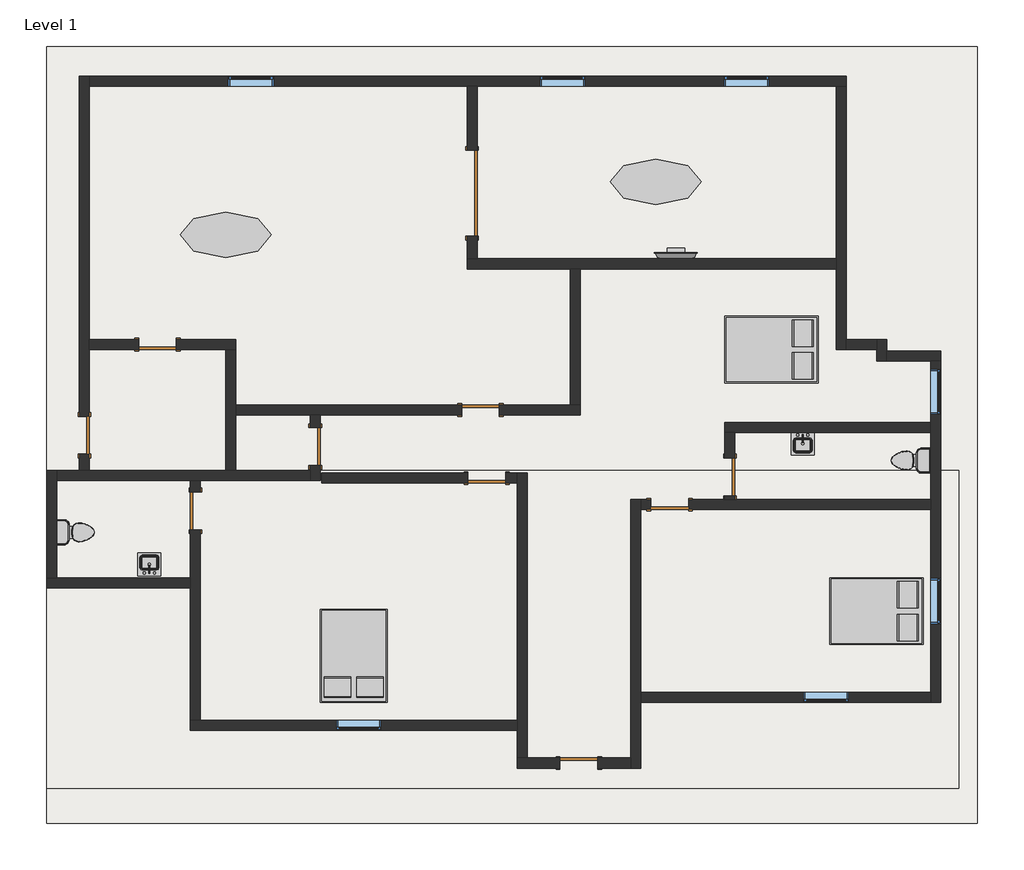
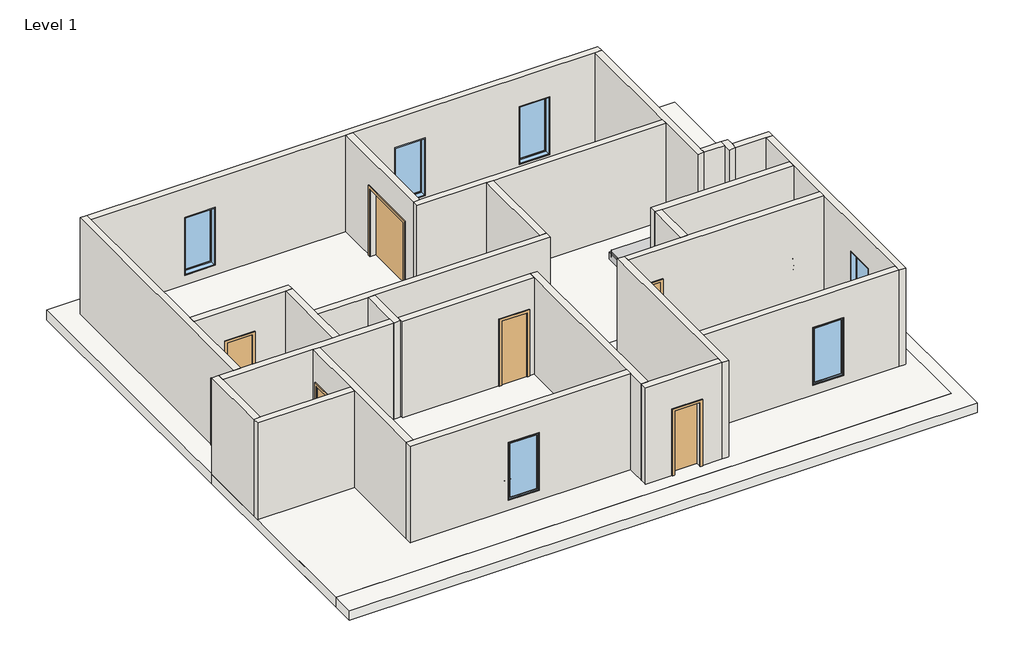
# One storey, incomplete: 27 walls, 10 doors, 7 windows, 6 furniture elements, 4 flow terminals, 3 slabs.
"""IFC4 building model written with IfcOpenShell, lengths in millimetres."""

from ifc_helpers import new_model, si_unit, frame, origin, origin_with_axes, place, context, project, spatial, polyline, outline, extrude, faceted_brep, transform, mapped, element, save
from components import door_f3de6620, door_53b1b562, door_fadea3f2, flow_terminal_871c2e40, toilet_domestic_3d_toilet_domestic_3d_f7549cf7, toilet_domestic_3d_toilet_domestic_3d_183bbd19, furniture_c8abb964, furniture_56245f3a, furniture_027a2ad9, window_9a779fa2, window_750da936

model = new_model("IFC4")

# Units and contexts
model_context = context("Model", 3, world=origin())
ifc_project = project(units=[si_unit("LENGTHUNIT", "METRE", prefix="MILLI")], contexts=[model_context])

# Site, building, storey
site = spatial("IfcSite", under=ifc_project)
building = spatial("IfcBuilding", under=site)
storey = spatial("IfcBuildingStorey", under=building, Name="Level 1", Elevation=0.0)

# Doors
placement = place(None, origin())
door_shape = door_f3de6620(model_context)
element("IfcDoor", 1, ObjectType="Door-Double-Flush_Panel-Double-Acting : 68\" x 84\"", at=placement, inside=storey, context=model_context, shape_type="MappedRepresentation", body=[
    mapped(door_shape, transform((-10205.5126434, 12193.5007235, 0.0), x_axis=(0.0, -1.0, 0.0), y_axis=(1.0, 0.0, 0.0), z_axis=(0.0, 0.0, 1.0))),
])
door_2_shape = door_53b1b562(model_context)
element("IfcDoor", 2, ObjectType="Single-Flush : 30\" x 80\"", at=placement, inside=storey, context=model_context, shape_type="MappedRepresentation", body=[
    mapped(door_2_shape, transform((-16538.7421908, 9145.5007235, 0.0), x_axis=(1.0, 0.0, 0.0), y_axis=(0.0, 1.0, 0.0), z_axis=(0.0, 0.0, 1.0))),
])
element("IfcDoor", 3, ObjectType="Single-Flush : 30\" x 80\"", at=placement, inside=storey, context=model_context, shape_type="MappedRepresentation", body=[
    mapped(door_2_shape, transform((-18011.9421908, 7316.7007235, 0.0), x_axis=(0.0, 1.0, 0.0), y_axis=(-1.0, 0.0, 0.0), z_axis=(0.0, 0.0, 1.0))),
])
element("IfcDoor", 4, ObjectType="Single-Flush : 30\" x 80\"", at=placement, inside=storey, context=model_context, shape_type="MappedRepresentation", body=[
    mapped(door_2_shape, transform((-9909.3421908, 6453.1007235, 0.0), x_axis=(1.0, 0.0, 0.0), y_axis=(0.0, 1.0, 0.0), z_axis=(0.0, 0.0, 1.0))),
])
element("IfcDoor", 5, ObjectType="Single-Flush : 30\" x 80\"", at=placement, inside=storey, context=model_context, shape_type="MappedRepresentation", body=[
    mapped(door_2_shape, transform((-8055.1421908, 712.7007235, 0.0), x_axis=(-1.0, 0.0, 0.0), y_axis=(0.0, -1.0, 0.0), z_axis=(0.0, 0.0, 1.0))),
])
door_3_shape = door_fadea3f2(model_context)
element("IfcDoor", 6, ObjectType="Single-Flush : 30\" x 80\"", at=placement, inside=storey, context=model_context, shape_type="MappedRepresentation", body=[
    mapped(door_3_shape, transform((-15776.7421908, 5792.7007235, 0.0), x_axis=(0.0, 1.0, 0.0), y_axis=(-1.0, 0.0, 0.0), z_axis=(0.0, 0.0, 1.0))),
])
element("IfcDoor", 7, ObjectType="Single-Flush : 30\" x 80\"", at=placement, inside=storey, context=model_context, shape_type="MappedRepresentation", body=[
    mapped(door_3_shape, transform((-13363.7421908, 7088.1007235, 0.0), x_axis=(0.0, -1.0, 0.0), y_axis=(1.0, 0.0, 0.0), z_axis=(0.0, 0.0, 1.0))),
])
element("IfcDoor", 8, ObjectType="Single-Flush : 30\" x 80\"", at=placement, inside=storey, context=model_context, shape_type="MappedRepresentation", body=[
    mapped(door_3_shape, transform((-10036.3421908, 7824.7007235, 0.0), x_axis=(1.0, 0.0, 0.0), y_axis=(0.0, 1.0, 0.0), z_axis=(0.0, 0.0, 1.0))),
])
element("IfcDoor", 9, ObjectType="Single-Flush : 30\" x 80\"", at=placement, inside=storey, context=model_context, shape_type="MappedRepresentation", body=[
    mapped(door_3_shape, transform((-6226.3421908, 5919.7007235, 0.0), x_axis=(-1.0, 0.0, 0.0), y_axis=(0.0, -1.0, 0.0), z_axis=(0.0, 0.0, 1.0))),
])
element("IfcDoor", 10, ObjectType="Single-Flush : 30\" x 80\"", at=placement, inside=storey, context=model_context, shape_type="MappedRepresentation", body=[
    mapped(door_3_shape, transform((-5014.2099629, 6478.5007235, 0.0), x_axis=(0.0, -1.0, 0.0), y_axis=(1.0, 0.0, 0.0), z_axis=(0.0, 0.0, 1.0))),
])

# Flow terminals
flow_terminal_shape = flow_terminal_871c2e40(model_context)
element("IfcFlowTerminal", 11, ObjectType="Sink Kitchen-Island : 18\" x 18\"", at=placement, inside=storey, context=model_context, shape_type="MappedRepresentation", body=[
    mapped(flow_terminal_shape, transform((-16688.1529503, 4715.5461246, 0.0), x_axis=(-1.0000000000000004, 0.0, 0.0), y_axis=(0.0, -1.0000000000000004, 0.0), z_axis=(0.0, 0.0, 1.0))),
])
element("IfcFlowTerminal", 12, ObjectType="Sink Kitchen-Island : 18\" x 18\"", at=placement, inside=storey, context=model_context, shape_type="MappedRepresentation", body=[
    mapped(flow_terminal_shape, transform((-3562.3314314, 7149.2553224, 0.0), x_axis=(1.0, 0.0, 0.0), y_axis=(0.0, 1.0, 0.0), z_axis=(0.0, 0.0, 1.0))),
])
toilet_domestic_3d_toilet_domestic_3d_shape = toilet_domestic_3d_toilet_domestic_3d_f7549cf7(model_context)
toilet_domestic_3d_toilet_domestic_3d_2_shape = toilet_domestic_3d_toilet_domestic_3d_183bbd19(model_context)
element("IfcFlowTerminal", 13, ObjectType="Toilet-Domestic-3D : Toilet-Domestic-3D", at=placement, inside=storey, context=model_context, shape_type="MappedRepresentation", body=[
    mapped(toilet_domestic_3d_toilet_domestic_3d_shape, transform((-18113.5421908, 5360.9007235, 0.0), x_axis=(0.0, 1.0000000000000002, 0.0), y_axis=(-1.0000000000000002, 0.0, 0.0), z_axis=(0.0, 0.0, 1.0))),
    mapped(toilet_domestic_3d_toilet_domestic_3d_2_shape, transform((-18113.5421908, 5360.9007235, 0.0), x_axis=(0.0, 1.0000000000000002, 0.0), y_axis=(-1.0000000000000002, 0.0, 0.0), z_axis=(0.0, 0.0, 1.0))),
])
element("IfcFlowTerminal", 14, ObjectType="Toilet-Domestic-3D : Toilet-Domestic-3D", at=placement, inside=storey, context=model_context, shape_type="MappedRepresentation", body=[
    mapped(toilet_domestic_3d_toilet_domestic_3d_shape, transform((-1463.2382182, 6808.7007235, 0.0), x_axis=(0.0, -1.0000000000000004, 0.0), y_axis=(1.0000000000000004, 0.0, 0.0), z_axis=(0.0, 0.0, 1.0))),
    mapped(toilet_domestic_3d_toilet_domestic_3d_2_shape, transform((-1463.2382182, 6808.7007235, 0.0), x_axis=(0.0, -1.0000000000000004, 0.0), y_axis=(1.0000000000000004, 0.0, 0.0), z_axis=(0.0, 0.0, 1.0))),
])

# Furniture
furniture_shape = furniture_c8abb964(model_context)
element("IfcFurniture", 15, ObjectType="Bed-Box : Double 53\" x 74\"", at=placement, inside=storey, context=model_context, shape_type="MappedRepresentation", body=[
    mapped(furniture_shape, transform((-12249.8897318, 2637.2712153, 0.0), x_axis=(-0.9999999999999999, 0.0, 0.0), y_axis=(0.0, -0.9999999999999999, 0.0), z_axis=(0.0, 0.0, 1.0))),
])
element("IfcFurniture", 16, ObjectType="Bed-Box : Double 53\" x 74\"", at=placement, inside=storey, context=model_context, shape_type="MappedRepresentation", body=[
    mapped(furniture_shape, transform((-1826.3126826, 4112.5531825, 0.0), x_axis=(0.0, -1.0000000000000002, 0.0), y_axis=(1.0000000000000002, 0.0, 0.0), z_axis=(0.0, 0.0, 1.0))),
])
element("IfcFurniture", 17, ObjectType="Bed-Box : Double 53\" x 74\"", at=placement, inside=storey, context=model_context, shape_type="MappedRepresentation", body=[
    mapped(furniture_shape, transform((-3941.5804547, 9383.0531825, 0.0), x_axis=(0.0, -0.9999999999999998, 0.0), y_axis=(0.9999999999999998, 0.0, 0.0), z_axis=(0.0, 0.0, 1.0))),
])
furniture_2_shape = furniture_56245f3a(model_context)
element("IfcFurniture", 18, ObjectType="TV - Flat Screen : 32\"", at=placement, inside=storey, context=model_context, shape_type="MappedRepresentation", body=[
    mapped(furniture_2_shape, transform((-6103.286705, 10931.2393472, 914.4), x_axis=(-0.9999999999999998, 0.0, 0.0), y_axis=(0.0, -0.9999999999999998, 0.0), z_axis=(0.0, 0.0, 1.0))),
])
furniture_3_shape = furniture_027a2ad9(model_context)
element("IfcFurniture", 19, ObjectType="Table-Ellipse : 72\" x 36\"", at=placement, inside=storey, context=model_context, shape_type="MappedRepresentation", body=[
    mapped(furniture_3_shape, transform((-15167.1421908, 11355.3007235, 0.0), x_axis=(1.0, 0.0, 0.0), y_axis=(0.0, 1.0, 0.0), z_axis=(0.0, 0.0, 1.0))),
])
element("IfcFurniture", 20, ObjectType="Table-Ellipse : 72\" x 36\"", at=placement, inside=storey, context=model_context, shape_type="MappedRepresentation", body=[
    mapped(furniture_3_shape, transform((-6505.7421908, 12422.1007235, 0.0), x_axis=(1.0, 0.0, 0.0), y_axis=(0.0, 1.0, 0.0), z_axis=(0.0, 0.0, 1.0))),
])

# Slabs
element("IfcSlab", 21, ObjectType="Generic - 12\"", at=placement, inside=storey, context=model_context, shape_type="SweptSolid", body=[
    extrude(outline(polyline([(-765.3421908, 14555.7007235), (-765.3421908, 6021.3007235), (-18113.5421908, 6021.3007235), (-18113.5421908, 14555.7007235), (-765.3421908, 14555.7007235)])), frame((0.0, 0.0, -304.8), z_axis=(0.0, 0.0, 1.0), x_axis=(1.0, 0.0, 0.0)), (0.0, 0.0, 1.0), 304.8),
])
element("IfcSlab", 22, ObjectType="Generic - 12\"", at=placement, inside=storey, context=model_context, shape_type="SweptSolid", body=[
    extrude(outline(polyline([(-409.7421908, 6605.5007235), (-409.7421908, 204.7007235), (-18773.9421908, 204.7007235), (-18773.9421908, 6605.5007235), (-409.7421908, 6605.5007235)])), frame((0.0, 0.0, -304.8), z_axis=(0.0, 0.0, 1.0), x_axis=(1.0, 0.0, 0.0)), (0.0, 0.0, 1.0), 304.8),
])
element("IfcSlab", 23, ObjectType="Generic - 12\"", at=placement, inside=storey, context=model_context, shape_type="SweptSolid", body=[
    extrude(outline(polyline([(-28.7421908, 15149.4135016), (-28.7421908, -496.9864984), (-18773.9421908, -496.9864984), (-18773.9421908, 15149.4135016), (-28.7421908, 15149.4135016)])), frame((0.0, 0.0, -304.8), z_axis=(0.0, 0.0, 1.0), x_axis=(1.0, 0.0, 0.0)), (0.0, 0.0, 1.0), 304.8),
])

# Walls
element("IfcWall", 24, ObjectType="Generic - 8\"", at=placement, inside=storey, context=model_context, shape_type="Brep", body=[
    faceted_brep([(-17910.3421908, 7697.7007235, 2032.0), (-17910.3421908, 7697.7007235, 0.0), (-17910.3421908, 9043.9007235, 0.0), (-17910.3421908, 9247.1007235, 0.0), (-17910.3421908, 14352.5007235, 0.0), (-17910.3421908, 14555.7007235, 0.0), (-17910.3421908, 14555.7007235, 3048.0), (-17910.3421908, 14352.5007235, 3048.0), (-17910.3421908, 9247.1007235, 3048.0), (-17910.3421908, 9043.9007235, 3048.0), (-17910.3421908, 6605.5007235, 3048.0), (-17910.3421908, 6605.5007235, 0.0), (-17910.3421908, 6935.7007235, 0.0), (-17910.3421908, 6935.7007235, 2032.0), (-18113.5421908, 14555.7007235, 0.0), (-18113.5421908, 7697.7007235, 0.0), (-18113.5421908, 7697.7007235, 2032.0), (-18113.5421908, 6935.7007235, 2032.0), (-18113.5421908, 6935.7007235, 0.0), (-18113.5421908, 6605.5007235, 0.0), (-18113.5421908, 6605.5007235, 3048.0), (-18113.5421908, 14555.7007235, 3048.0)], [[[0, 1, 2, 3, 4, 5, 6, 7, 8, 9, 10, 11, 12, 13]], [[14, 15, 16, 17, 18, 19, 20, 21]], [[12, 11, 19, 18]], [[5, 4, 3, 2, 1, 15, 14]], [[6, 5, 14, 21]], [[11, 10, 20, 19]], [[16, 15, 1, 0]], [[17, 16, 0, 13]], [[18, 17, 13, 12]], [[10, 9, 8, 7, 6, 21, 20]]]),
])
element("IfcWall", 25, ObjectType="Generic - 8\"", at=placement, inside=storey, context=model_context, shape_type="Brep", body=[
    faceted_brep([(-17910.3421908, 14352.5007235, 0.0), (-10307.1126434, 14352.5007235, 0.0), (-10103.9126434, 14352.5007235, 0.0), (-2873.5421908, 14352.5007235, 0.0), (-2670.3421908, 14352.5007235, 0.0), (-2670.3421908, 14352.5007235, 3048.0), (-2873.5421908, 14352.5007235, 3048.0), (-10103.9126434, 14352.5007235, 3048.0), (-10307.1126434, 14352.5007235, 3048.0), (-17910.3421908, 14352.5007235, 3048.0), (-14201.9421908, 14352.5007235, 2133.6), (-14201.9421908, 14352.5007235, 304.8), (-15116.3421908, 14352.5007235, 304.8), (-15116.3421908, 14352.5007235, 2133.6), (-8842.5421908, 14352.5007235, 2133.6), (-7928.1421908, 14352.5007235, 2133.6), (-7928.1421908, 14352.5007235, 304.8), (-8842.5421908, 14352.5007235, 304.8), (-4219.7421908, 14352.5007235, 2133.6), (-4219.7421908, 14352.5007235, 304.8), (-5134.1421908, 14352.5007235, 304.8), (-5134.1421908, 14352.5007235, 2133.6), (-17910.3421908, 14555.7007235, 0.0), (-17910.3421908, 14555.7007235, 3048.0), (-2670.3421908, 14555.7007235, 3048.0), (-2670.3421908, 14555.7007235, 0.0), (-14201.9421908, 14555.7007235, 2133.6), (-15116.3421908, 14555.7007235, 2133.6), (-15116.3421908, 14555.7007235, 304.8), (-14201.9421908, 14555.7007235, 304.8), (-8842.5421908, 14555.7007235, 2133.6), (-8842.5421908, 14555.7007235, 304.8), (-7928.1421908, 14555.7007235, 304.8), (-7928.1421908, 14555.7007235, 2133.6), (-4219.7421908, 14555.7007235, 2133.6), (-5134.1421908, 14555.7007235, 2133.6), (-5134.1421908, 14555.7007235, 304.8), (-4219.7421908, 14555.7007235, 304.8)], [[[0, 1, 2, 3, 4, 5, 6, 7, 8, 9], [10, 11, 12, 13], [14, 15, 16, 17], [18, 19, 20, 21]], [[22, 23, 24, 25], [26, 27, 28, 29], [30, 31, 32, 33], [34, 35, 36, 37]], [[4, 3, 2, 1, 0, 22, 25]], [[0, 9, 23, 22]], [[5, 4, 25, 24]], [[11, 10, 26, 29]], [[12, 11, 29, 28]], [[13, 12, 28, 27]], [[10, 13, 27, 26]], [[31, 30, 14, 17]], [[32, 31, 17, 16]], [[33, 32, 16, 15]], [[30, 33, 15, 14]], [[19, 18, 34, 37]], [[20, 19, 37, 36]], [[21, 20, 36, 35]], [[18, 21, 35, 34]], [[9, 8, 7, 6, 5, 24, 23]]]),
])
element("IfcWall", 26, ObjectType="Generic - 8\"", at=placement, inside=storey, context=model_context, shape_type="Brep", body=[
    faceted_brep([(-2873.5421908, 14352.5007235, 0.0), (-2873.5421908, 10872.7007235, 0.0), (-2873.5421908, 10669.5007235, 0.0), (-2873.5421908, 9043.9007235, 0.0), (-2873.5421908, 9043.9007235, 3048.0), (-2873.5421908, 10669.5007235, 3048.0), (-2873.5421908, 10872.7007235, 3048.0), (-2873.5421908, 14352.5007235, 3048.0), (-2670.3421908, 14352.5007235, 0.0), (-2670.3421908, 14352.5007235, 3048.0), (-2670.3421908, 9247.1007235, 3048.0), (-2670.3421908, 9043.9007235, 3048.0), (-2670.3421908, 9043.9007235, 0.0), (-2670.3421908, 9247.1007235, 0.0)], [[[0, 1, 2, 3, 4, 5, 6, 7]], [[8, 9, 10, 11, 12, 13]], [[3, 2, 1, 0, 8, 13, 12]], [[0, 7, 9, 8]], [[4, 3, 12, 11]], [[7, 6, 5, 4, 11, 10, 9]]]),
])
element("IfcWall", 27, ObjectType="Generic - 8\"", at=placement, inside=storey, context=model_context, shape_type="SweptSolid", body=[
    extrude(outline(polyline([(-2060.7421908, 9043.9007235), (-2670.3421908, 9043.9007235), (-2670.3421908, 9247.1007235), (-2060.7421908, 9247.1007235), (-2060.7421908, 9043.9007235)])), origin_with_axes(), (0.0, 0.0, 1.0), 3048.0),
])
element("IfcWall", 28, ObjectType="Generic - 8\"", at=placement, inside=storey, context=model_context, shape_type="Brep", body=[
    faceted_brep([(-2060.7421908, 9247.1007235, 0.0), (-2060.7421908, 9043.9007235, 0.0), (-2060.7421908, 8815.3007235, 0.0), (-2060.7421908, 8815.3007235, 3048.0), (-2060.7421908, 9043.9007235, 3048.0), (-2060.7421908, 9247.1007235, 3048.0), (-1857.5421908, 9247.1007235, 0.0), (-1857.5421908, 9247.1007235, 3048.0), (-1857.5421908, 9018.5007235, 3048.0), (-1857.5421908, 8815.3007235, 3048.0), (-1857.5421908, 8815.3007235, 0.0), (-1857.5421908, 9018.5007235, 0.0)], [[[0, 1, 2, 3, 4, 5]], [[6, 7, 8, 9, 10, 11]], [[2, 1, 0, 6, 11, 10]], [[0, 5, 7, 6]], [[3, 2, 10, 9]], [[5, 4, 3, 9, 8, 7]]]),
])
element("IfcWall", 29, ObjectType="Generic - 8\"", at=placement, inside=storey, context=model_context, shape_type="Brep", body=[
    faceted_brep([(-1857.5421908, 8815.3007235, 0.0), (-968.5421908, 8815.3007235, 0.0), (-765.3421908, 8815.3007235, 0.0), (-765.3421908, 8815.3007235, 3048.0), (-968.5421908, 8815.3007235, 3048.0), (-1857.5421908, 8815.3007235, 3048.0), (-1857.5421908, 9018.5007235, 0.0), (-1857.5421908, 9018.5007235, 3048.0), (-765.3421908, 9018.5007235, 3048.0), (-765.3421908, 9018.5007235, 0.0)], [[[0, 1, 2, 3, 4, 5]], [[6, 7, 8, 9]], [[2, 1, 0, 6, 9]], [[0, 5, 7, 6]], [[3, 2, 9, 8]], [[5, 4, 3, 8, 7]]]),
])
element("IfcWall", 30, ObjectType="Generic - 8\"", at=placement, inside=storey, context=model_context, shape_type="Brep", body=[
    faceted_brep([(-968.5421908, 8815.3007235, 0.0), (-968.5421908, 7570.7007235, 0.0), (-968.5421908, 7367.5007235, 0.0), (-968.5421908, 6021.3007235, 0.0), (-968.5421908, 5818.1007235, 0.0), (-968.5421908, 2135.1007235, 0.0), (-968.5421908, 1931.9007235, 0.0), (-968.5421908, 1931.9007235, 3048.0), (-968.5421908, 2135.1007235, 3048.0), (-968.5421908, 5818.1007235, 3048.0), (-968.5421908, 6021.3007235, 3048.0), (-968.5421908, 7367.5007235, 3048.0), (-968.5421908, 7570.7007235, 3048.0), (-968.5421908, 8815.3007235, 3048.0), (-968.5421908, 7735.8007235, 2133.6), (-968.5421908, 7735.8007235, 304.8), (-968.5421908, 8650.2007235, 304.8), (-968.5421908, 8650.2007235, 2133.6), (-968.5421908, 3519.4007235, 2133.6), (-968.5421908, 3519.4007235, 304.8), (-968.5421908, 4433.8007235, 304.8), (-968.5421908, 4433.8007235, 2133.6), (-765.3421908, 8815.3007235, 0.0), (-765.3421908, 8815.3007235, 3048.0), (-765.3421908, 1931.9007235, 3048.0), (-765.3421908, 1931.9007235, 0.0), (-765.3421908, 7735.8007235, 2133.6), (-765.3421908, 8650.2007235, 2133.6), (-765.3421908, 8650.2007235, 304.8), (-765.3421908, 7735.8007235, 304.8), (-765.3421908, 3519.4007235, 2133.6), (-765.3421908, 4433.8007235, 2133.6), (-765.3421908, 4433.8007235, 304.8), (-765.3421908, 3519.4007235, 304.8)], [[[0, 1, 2, 3, 4, 5, 6, 7, 8, 9, 10, 11, 12, 13], [14, 15, 16, 17], [18, 19, 20, 21]], [[22, 23, 24, 25], [26, 27, 28, 29], [30, 31, 32, 33]], [[6, 5, 4, 3, 2, 1, 0, 22, 25]], [[0, 13, 23, 22]], [[7, 6, 25, 24]], [[15, 14, 26, 29]], [[16, 15, 29, 28]], [[17, 16, 28, 27]], [[14, 17, 27, 26]], [[19, 18, 30, 33]], [[20, 19, 33, 32]], [[21, 20, 32, 31]], [[18, 21, 31, 30]], [[13, 12, 11, 10, 9, 8, 7, 24, 23]]]),
])
element("IfcWall", 31, ObjectType="Generic - 8\"", at=placement, inside=storey, context=model_context, shape_type="SweptSolid", body=[
    extrude(outline(polyline([(0.0, -968.5421908), (3048.0, -968.5421908), (3048.0, -6810.5421908), (0.0, -6810.5421908), (0.0, -968.5421908)]), holes=[polyline([(2133.6, -3533.9421908), (2133.6, -2619.5421908), (304.8, -2619.5421908), (304.8, -3533.9421908), (2133.6, -3533.9421908)])]), frame((0.0, 1931.9007235, 0.0), z_axis=(0.0, 1.0, 0.0), x_axis=(0.0, 0.0, 1.0)), (0.0, 0.0, 1.0), 203.2),
])
element("IfcWall", 32, ObjectType="Generic - 8\"", at=placement, inside=storey, context=model_context, shape_type="Brep", body=[
    faceted_brep([(-7013.7421908, 6021.3007235, 0.0), (-7013.7421908, 814.3007235, 0.0), (-7013.7421908, 611.1007235, 0.0), (-7013.7421908, 611.1007235, 3048.0), (-7013.7421908, 814.3007235, 3048.0), (-7013.7421908, 6021.3007235, 3048.0), (-6810.5421908, 6021.3007235, 0.0), (-6810.5421908, 6021.3007235, 3048.0), (-6810.5421908, 5818.1007235, 3048.0), (-6810.5421908, 2135.1007235, 3048.0), (-6810.5421908, 1931.9007235, 3048.0), (-6810.5421908, 611.1007235, 3048.0), (-6810.5421908, 611.1007235, 0.0), (-6810.5421908, 1931.9007235, 0.0), (-6810.5421908, 2135.1007235, 0.0), (-6810.5421908, 5818.1007235, 0.0)], [[[0, 1, 2, 3, 4, 5]], [[6, 7, 8, 9, 10, 11, 12, 13, 14, 15]], [[2, 1, 0, 6, 15, 14, 13, 12]], [[3, 2, 12, 11]], [[0, 5, 7, 6]], [[5, 4, 3, 11, 10, 9, 8, 7]]]),
])
element("IfcWall", 33, ObjectType="Generic - 8\"", at=placement, inside=storey, context=model_context, shape_type="Brep", body=[
    faceted_brep([(-8436.1421908, 814.3007235, 2032.0), (-8436.1421908, 814.3007235, 0.0), (-9096.5421908, 814.3007235, 0.0), (-9299.7421908, 814.3007235, 0.0), (-9299.7421908, 814.3007235, 3048.0), (-9096.5421908, 814.3007235, 3048.0), (-7013.7421908, 814.3007235, 3048.0), (-7013.7421908, 814.3007235, 0.0), (-7674.1421908, 814.3007235, 0.0), (-7674.1421908, 814.3007235, 2032.0), (-9299.7421908, 611.1007235, 0.0), (-8436.1421908, 611.1007235, 0.0), (-8436.1421908, 611.1007235, 2032.0), (-7674.1421908, 611.1007235, 2032.0), (-7674.1421908, 611.1007235, 0.0), (-7013.7421908, 611.1007235, 0.0), (-7013.7421908, 611.1007235, 3048.0), (-9299.7421908, 611.1007235, 3048.0)], [[[0, 1, 2, 3, 4, 5, 6, 7, 8, 9]], [[10, 11, 12, 13, 14, 15, 16, 17]], [[8, 7, 15, 14]], [[3, 2, 1, 11, 10]], [[7, 6, 16, 15]], [[4, 3, 10, 17]], [[12, 11, 1, 0]], [[13, 12, 0, 9]], [[14, 13, 9, 8]], [[6, 5, 4, 17, 16]]]),
])
element("IfcWall", 34, ObjectType="Generic - 8\"", at=placement, inside=storey, context=model_context, shape_type="Brep", body=[
    faceted_brep([(-9096.5421908, 814.3007235, 0.0), (-9096.5421908, 6554.7007235, 0.0), (-9096.5421908, 6554.7007235, 3048.0), (-9096.5421908, 814.3007235, 3048.0), (-9299.7421908, 814.3007235, 0.0), (-9299.7421908, 814.3007235, 3048.0), (-9299.7421908, 1373.1007235, 3048.0), (-9299.7421908, 1576.3007235, 3048.0), (-9299.7421908, 6351.5007235, 3048.0), (-9299.7421908, 6554.7007235, 3048.0), (-9299.7421908, 6554.7007235, 0.0), (-9299.7421908, 6351.5007235, 0.0), (-9299.7421908, 1576.3007235, 0.0), (-9299.7421908, 1373.1007235, 0.0)], [[[0, 1, 2, 3]], [[4, 5, 6, 7, 8, 9, 10, 11, 12, 13]], [[1, 0, 4, 13, 12, 11, 10]], [[0, 3, 5, 4]], [[2, 1, 10, 9]], [[3, 2, 9, 8, 7, 6, 5]]]),
])
element("IfcWall", 35, ObjectType="Generic - 8\"", at=placement, inside=storey, context=model_context, shape_type="Brep", body=[
    faceted_brep([(-9299.7421908, 1576.3007235, 0.0), (-15675.1421908, 1576.3007235, 0.0), (-15878.3421908, 1576.3007235, 0.0), (-15878.3421908, 1576.3007235, 3048.0), (-15675.1421908, 1576.3007235, 3048.0), (-9299.7421908, 1576.3007235, 3048.0), (-12944.6421908, 1576.3007235, 2133.6), (-12944.6421908, 1576.3007235, 304.8), (-12030.2421908, 1576.3007235, 304.8), (-12030.2421908, 1576.3007235, 2133.6), (-9299.7421908, 1373.1007235, 0.0), (-9299.7421908, 1373.1007235, 3048.0), (-15878.3421908, 1373.1007235, 3048.0), (-15878.3421908, 1373.1007235, 0.0), (-12944.6421908, 1373.1007235, 2133.6), (-12030.2421908, 1373.1007235, 2133.6), (-12030.2421908, 1373.1007235, 304.8), (-12944.6421908, 1373.1007235, 304.8)], [[[0, 1, 2, 3, 4, 5], [6, 7, 8, 9]], [[10, 11, 12, 13], [14, 15, 16, 17]], [[2, 1, 0, 10, 13]], [[0, 5, 11, 10]], [[3, 2, 13, 12]], [[7, 6, 14, 17]], [[8, 7, 17, 16]], [[9, 8, 16, 15]], [[6, 9, 15, 14]], [[5, 4, 3, 12, 11]]]),
])
element("IfcWall", 36, ObjectType="Generic - 8\"", at=placement, inside=storey, context=model_context, shape_type="Brep", body=[
    faceted_brep([(-15675.1421908, 6173.7007235, 2032.0), (-15675.1421908, 6173.7007235, 0.0), (-15675.1421908, 6402.3007235, 0.0), (-15675.1421908, 6402.3007235, 3048.0), (-15675.1421908, 1576.3007235, 3048.0), (-15675.1421908, 1576.3007235, 0.0), (-15675.1421908, 5411.7007235, 0.0), (-15675.1421908, 5411.7007235, 2032.0), (-15878.3421908, 6402.3007235, 0.0), (-15878.3421908, 6173.7007235, 0.0), (-15878.3421908, 6173.7007235, 2032.0), (-15878.3421908, 5411.7007235, 2032.0), (-15878.3421908, 5411.7007235, 0.0), (-15878.3421908, 4446.5007235, 0.0), (-15878.3421908, 4243.3007235, 0.0), (-15878.3421908, 1576.3007235, 0.0), (-15878.3421908, 1576.3007235, 3048.0), (-15878.3421908, 4243.3007235, 3048.0), (-15878.3421908, 4446.5007235, 3048.0), (-15878.3421908, 6402.3007235, 3048.0)], [[[0, 1, 2, 3, 4, 5, 6, 7]], [[8, 9, 10, 11, 12, 13, 14, 15, 16, 17, 18, 19]], [[6, 5, 15, 14, 13, 12]], [[2, 1, 9, 8]], [[5, 4, 16, 15]], [[3, 2, 8, 19]], [[10, 9, 1, 0]], [[11, 10, 0, 7]], [[12, 11, 7, 6]], [[4, 3, 19, 18, 17, 16]]]),
])
element("IfcWall", 37, ObjectType="Generic - 8\"", at=placement, inside=storey, context=model_context, shape_type="Brep", body=[
    faceted_brep([(-15878.3421908, 4446.5007235, 0.0), (-18570.7421908, 4446.5007235, 0.0), (-18773.9421908, 4446.5007235, 0.0), (-18773.9421908, 4446.5007235, 3048.0), (-18570.7421908, 4446.5007235, 3048.0), (-15878.3421908, 4446.5007235, 3048.0), (-15878.3421908, 4243.3007235, 0.0), (-15878.3421908, 4243.3007235, 3048.0), (-18773.9421908, 4243.3007235, 3048.0), (-18773.9421908, 4243.3007235, 0.0)], [[[0, 1, 2, 3, 4, 5]], [[6, 7, 8, 9]], [[2, 1, 0, 6, 9]], [[0, 5, 7, 6]], [[3, 2, 9, 8]], [[5, 4, 3, 8, 7]]]),
])
element("IfcWall", 38, ObjectType="Generic - 8\"", at=placement, inside=storey, context=model_context, shape_type="Brep", body=[
    faceted_brep([(-18570.7421908, 4446.5007235, 0.0), (-18570.7421908, 6402.3007235, 0.0), (-18570.7421908, 6605.5007235, 0.0), (-18570.7421908, 6605.5007235, 3048.0), (-18570.7421908, 6402.3007235, 3048.0), (-18570.7421908, 4446.5007235, 3048.0), (-18773.9421908, 4446.5007235, 0.0), (-18773.9421908, 4446.5007235, 3048.0), (-18773.9421908, 6605.5007235, 3048.0), (-18773.9421908, 6605.5007235, 0.0)], [[[0, 1, 2, 3, 4, 5]], [[6, 7, 8, 9]], [[2, 1, 0, 6, 9]], [[0, 5, 7, 6]], [[3, 2, 9, 8]], [[5, 4, 3, 8, 7]]]),
])
element("IfcWall", 39, ObjectType="Generic - 8\"", at=placement, inside=storey, context=model_context, shape_type="Brep", body=[
    faceted_brep([(-18570.7421908, 6402.3007235, 0.0), (-15878.3421908, 6402.3007235, 0.0), (-15675.1421908, 6402.3007235, 0.0), (-13465.3421908, 6402.3007235, 0.0), (-13465.3421908, 6402.3007235, 3048.0), (-15675.1421908, 6402.3007235, 3048.0), (-15878.3421908, 6402.3007235, 3048.0), (-18570.7421908, 6402.3007235, 3048.0), (-18570.7421908, 6605.5007235, 0.0), (-18570.7421908, 6605.5007235, 3048.0), (-18113.5421908, 6605.5007235, 3048.0), (-17910.3421908, 6605.5007235, 3048.0), (-15167.1421908, 6605.5007235, 3048.0), (-14963.9421908, 6605.5007235, 3048.0), (-13465.3421908, 6605.5007235, 3048.0), (-13465.3421908, 6605.5007235, 0.0), (-14963.9421908, 6605.5007235, 0.0), (-15167.1421908, 6605.5007235, 0.0), (-17910.3421908, 6605.5007235, 0.0), (-18113.5421908, 6605.5007235, 0.0)], [[[0, 1, 2, 3, 4, 5, 6, 7]], [[8, 9, 10, 11, 12, 13, 14, 15, 16, 17, 18, 19]], [[3, 2, 1, 0, 8, 19, 18, 17, 16, 15]], [[0, 7, 9, 8]], [[4, 3, 15, 14]], [[7, 6, 5, 4, 14, 13, 12, 11, 10, 9]]]),
])
element("IfcWall", 40, ObjectType="Generic - 8\"", at=placement, inside=storey, context=model_context, shape_type="Brep", body=[
    faceted_brep([(-10307.1126434, 10669.5007235, 0.0), (-8232.9421908, 10669.5007235, 0.0), (-8029.7421908, 10669.5007235, 0.0), (-2873.5421908, 10669.5007235, 0.0), (-2873.5421908, 10669.5007235, 3048.0), (-8029.7421908, 10669.5007235, 3048.0), (-8232.9421908, 10669.5007235, 3048.0), (-10307.1126434, 10669.5007235, 3048.0), (-10307.1126434, 10872.7007235, 0.0), (-10307.1126434, 10872.7007235, 3048.0), (-10103.9126434, 10872.7007235, 3048.0), (-2873.5421908, 10872.7007235, 3048.0), (-2873.5421908, 10872.7007235, 0.0), (-10103.9126434, 10872.7007235, 0.0)], [[[0, 1, 2, 3, 4, 5, 6, 7]], [[8, 9, 10, 11, 12, 13]], [[3, 2, 1, 0, 8, 13, 12]], [[4, 3, 12, 11]], [[0, 7, 9, 8]], [[7, 6, 5, 4, 11, 10, 9]]]),
])
element("IfcWall", 41, ObjectType="Generic - 8\"", at=placement, inside=storey, context=model_context, shape_type="Brep", body=[
    faceted_brep([(-16157.7421908, 9043.9007235, 2032.0), (-16157.7421908, 9043.9007235, 0.0), (-15167.1421908, 9043.9007235, 0.0), (-14963.9421908, 9043.9007235, 0.0), (-14963.9421908, 9043.9007235, 3048.0), (-15167.1421908, 9043.9007235, 3048.0), (-17910.3421908, 9043.9007235, 3048.0), (-17910.3421908, 9043.9007235, 0.0), (-16919.7421908, 9043.9007235, 0.0), (-16919.7421908, 9043.9007235, 2032.0), (-14963.9421908, 9247.1007235, 0.0), (-16157.7421908, 9247.1007235, 0.0), (-16157.7421908, 9247.1007235, 2032.0), (-16919.7421908, 9247.1007235, 2032.0), (-16919.7421908, 9247.1007235, 0.0), (-17910.3421908, 9247.1007235, 0.0), (-17910.3421908, 9247.1007235, 3048.0), (-14963.9421908, 9247.1007235, 3048.0)], [[[0, 1, 2, 3, 4, 5, 6, 7, 8, 9]], [[10, 11, 12, 13, 14, 15, 16, 17]], [[8, 7, 15, 14]], [[3, 2, 1, 11, 10]], [[7, 6, 16, 15]], [[4, 3, 10, 17]], [[12, 11, 1, 0]], [[13, 12, 0, 9]], [[14, 13, 9, 8]], [[6, 5, 4, 17, 16]]]),
])
element("IfcWall", 42, ObjectType="Generic - 8\"", at=placement, inside=storey, context=model_context, shape_type="Brep", body=[
    faceted_brep([(-15167.1421908, 9043.9007235, 0.0), (-15167.1421908, 6605.5007235, 0.0), (-15167.1421908, 6605.5007235, 3048.0), (-15167.1421908, 9043.9007235, 3048.0), (-14963.9421908, 9043.9007235, 0.0), (-14963.9421908, 9043.9007235, 3048.0), (-14963.9421908, 7926.3007235, 3048.0), (-14963.9421908, 7723.1007235, 3048.0), (-14963.9421908, 6605.5007235, 3048.0), (-14963.9421908, 6605.5007235, 0.0), (-14963.9421908, 7723.1007235, 0.0), (-14963.9421908, 7926.3007235, 0.0)], [[[0, 1, 2, 3]], [[4, 5, 6, 7, 8, 9, 10, 11]], [[1, 0, 4, 11, 10, 9]], [[0, 3, 5, 4]], [[2, 1, 9, 8]], [[3, 2, 8, 7, 6, 5]]]),
])
element("IfcWall", 43, ObjectType="Generic - 8\"", at=placement, inside=storey, context=model_context, shape_type="Brep", body=[
    faceted_brep([(-9655.3421908, 7723.1007235, 2032.0), (-9655.3421908, 7723.1007235, 0.0), (-8029.7421908, 7723.1007235, 0.0), (-8029.7421908, 7723.1007235, 3048.0), (-13262.1421908, 7723.1007235, 3048.0), (-13465.3421908, 7723.1007235, 3048.0), (-14963.9421908, 7723.1007235, 3048.0), (-14963.9421908, 7723.1007235, 0.0), (-13465.3421908, 7723.1007235, 0.0), (-13262.1421908, 7723.1007235, 0.0), (-10417.3421908, 7723.1007235, 0.0), (-10417.3421908, 7723.1007235, 2032.0), (-8029.7421908, 7926.3007235, 0.0), (-8232.9421908, 7926.3007235, 0.0), (-9655.3421908, 7926.3007235, 0.0), (-9655.3421908, 7926.3007235, 2032.0), (-10417.3421908, 7926.3007235, 2032.0), (-10417.3421908, 7926.3007235, 0.0), (-14963.9421908, 7926.3007235, 0.0), (-14963.9421908, 7926.3007235, 3048.0), (-8232.9421908, 7926.3007235, 3048.0), (-8029.7421908, 7926.3007235, 3048.0)], [[[0, 1, 2, 3, 4, 5, 6, 7, 8, 9, 10, 11]], [[12, 13, 14, 15, 16, 17, 18, 19, 20, 21]], [[2, 1, 14, 13, 12]], [[10, 9, 8, 7, 18, 17]], [[7, 6, 19, 18]], [[3, 2, 12, 21]], [[15, 14, 1, 0]], [[16, 15, 0, 11]], [[17, 16, 11, 10]], [[6, 5, 4, 3, 21, 20, 19]]]),
])
element("IfcWall", 44, ObjectType="Generic - 8\"", at=placement, inside=storey, context=model_context, shape_type="SweptSolid", body=[
    extrude(outline(polyline([(-8029.7421908, 10669.5007235), (-8029.7421908, 7926.3007235), (-8232.9421908, 7926.3007235), (-8232.9421908, 10669.5007235), (-8029.7421908, 10669.5007235)])), origin_with_axes(), (0.0, 0.0, 1.0), 3048.0),
])
element("IfcWall", 45, ObjectType="Generic - 8\"", at=placement, inside=storey, context=model_context, shape_type="Brep", body=[
    faceted_brep([(-6810.5421908, 5818.1007235, 0.0), (-6607.3421908, 5818.1007235, 0.0), (-6607.3421908, 5818.1007235, 2032.0), (-5845.3421908, 5818.1007235, 2032.0), (-5845.3421908, 5818.1007235, 0.0), (-968.5421908, 5818.1007235, 0.0), (-968.5421908, 5818.1007235, 3048.0), (-6810.5421908, 5818.1007235, 3048.0), (-6607.3421908, 6021.3007235, 2032.0), (-6607.3421908, 6021.3007235, 0.0), (-6810.5421908, 6021.3007235, 0.0), (-6810.5421908, 6021.3007235, 3048.0), (-5115.8099629, 6021.3007235, 3048.0), (-4912.6099629, 6021.3007235, 3048.0), (-968.5421908, 6021.3007235, 3048.0), (-968.5421908, 6021.3007235, 0.0), (-4912.6099629, 6021.3007235, 0.0), (-5115.8099629, 6021.3007235, 0.0), (-5845.3421908, 6021.3007235, 0.0), (-5845.3421908, 6021.3007235, 2032.0)], [[[0, 1, 2, 3, 4, 5, 6, 7]], [[8, 9, 10, 11, 12, 13, 14, 15, 16, 17, 18, 19]], [[10, 9, 1, 0]], [[18, 17, 16, 15, 5, 4]], [[0, 7, 11, 10]], [[6, 5, 15, 14]], [[2, 1, 9, 8]], [[3, 2, 8, 19]], [[4, 3, 19, 18]], [[7, 6, 14, 13, 12, 11]]]),
])
element("IfcWall", 46, ObjectType="Generic - 8\"", at=placement, inside=storey, context=model_context, shape_type="Brep", body=[
    faceted_brep([(-13262.1421908, 6402.3007235, 0.0), (-13262.1421908, 6707.1007235, 0.0), (-13262.1421908, 6707.1007235, 2032.0), (-13262.1421908, 7469.1007235, 2032.0), (-13262.1421908, 7469.1007235, 0.0), (-13262.1421908, 7723.1007235, 0.0), (-13262.1421908, 7723.1007235, 3048.0), (-13262.1421908, 6402.3007235, 3048.0), (-13465.3421908, 6707.1007235, 2032.0), (-13465.3421908, 6707.1007235, 0.0), (-13465.3421908, 6605.5007235, 0.0), (-13465.3421908, 6402.3007235, 0.0), (-13465.3421908, 6402.3007235, 3048.0), (-13465.3421908, 6605.5007235, 3048.0), (-13465.3421908, 7723.1007235, 3048.0), (-13465.3421908, 7723.1007235, 0.0), (-13465.3421908, 7469.1007235, 0.0), (-13465.3421908, 7469.1007235, 2032.0)], [[[0, 1, 2, 3, 4, 5, 6, 7]], [[8, 9, 10, 11, 12, 13, 14, 15, 16, 17]], [[16, 15, 5, 4]], [[11, 10, 9, 1, 0]], [[6, 5, 15, 14]], [[2, 1, 9, 8]], [[3, 2, 8, 17]], [[4, 3, 17, 16]], [[0, 7, 12, 11]], [[7, 6, 14, 13, 12]]]),
])
element("IfcWall", 47, ObjectType="Generic - 8\"", at=placement, inside=storey, context=model_context, shape_type="SweptSolid", body=[
    extrude(outline(polyline([(2032.0, -9528.3421908), (0.0, -9528.3421908), (0.0, -9299.7421908), (3048.0, -9299.7421908), (3048.0, -13236.7421908), (0.0, -13236.7421908), (0.0, -10290.3421908), (2032.0, -10290.3421908), (2032.0, -9528.3421908)])), frame((0.0, 6351.5007235, 0.0), z_axis=(0.0, 1.0, 0.0), x_axis=(0.0, 0.0, 1.0)), (0.0, 0.0, 1.0), 203.2),
])
element("IfcWall", 48, ObjectType="Generic - 8\"", at=placement, inside=storey, context=model_context, shape_type="Brep", body=[
    faceted_brep([(-968.5421908, 7570.7007235, 0.0), (-5115.8099629, 7570.7007235, 0.0), (-5115.8099629, 7570.7007235, 3048.0), (-968.5421908, 7570.7007235, 3048.0), (-968.5421908, 7367.5007235, 0.0), (-968.5421908, 7367.5007235, 3048.0), (-4912.6099629, 7367.5007235, 3048.0), (-5115.8099629, 7367.5007235, 3048.0), (-5115.8099629, 7367.5007235, 0.0), (-4912.6099629, 7367.5007235, 0.0)], [[[0, 1, 2, 3]], [[4, 5, 6, 7, 8, 9]], [[1, 0, 4, 9, 8]], [[0, 3, 5, 4]], [[2, 1, 8, 7]], [[3, 2, 7, 6, 5]]]),
])
element("IfcWall", 49, ObjectType="Generic - 8\"", at=placement, inside=storey, context=model_context, shape_type="SweptSolid", body=[
    extrude(outline(polyline([(6097.5007235, 2032.0), (6097.5007235, 0.0), (6021.3007235, 0.0), (6021.3007235, 3048.0), (7367.5007235, 3048.0), (7367.5007235, 0.0), (6859.5007235, 0.0), (6859.5007235, 2032.0), (6097.5007235, 2032.0)])), frame((-5115.8099629, 0.0, 0.0), z_axis=(1.0, 0.0, 0.0), x_axis=(0.0, 1.0, 0.0)), (0.0, 0.0, 1.0), 203.2),
])
element("IfcWall", 50, ObjectType="Generic - 8\"", at=placement, inside=storey, context=model_context, shape_type="SweptSolid", body=[
    extrude(outline(polyline([(10872.7007235, 0.0), (10872.7007235, 3048.0), (14352.5007235, 3048.0), (14352.5007235, 0.0), (13057.1007235, 0.0), (13057.1007235, 2133.6), (11329.9007235, 2133.6), (11329.9007235, 0.0), (10872.7007235, 0.0)])), frame((-10307.1126434, 0.0, 0.0), z_axis=(1.0, 0.0, 0.0), x_axis=(0.0, 1.0, 0.0)), (0.0, 0.0, 1.0), 203.2),
])

# Windows
window_shape = window_9a779fa2(model_context)
element("IfcWindow", 51, ObjectType="Fixed : 36\" x 72\"", at=placement, inside=storey, context=model_context, shape_type="MappedRepresentation", body=[
    mapped(window_shape, transform((-14621.0421908, 14454.1007235, 0.0), x_axis=(1.0, 0.0, 0.0), y_axis=(0.0, 1.0, 0.0), z_axis=(0.0, 0.0, 1.0))),
])
element("IfcWindow", 52, ObjectType="Fixed : 36\" x 72\"", at=placement, inside=storey, context=model_context, shape_type="MappedRepresentation", body=[
    mapped(window_shape, transform((-4638.8421908, 14454.1007235, 0.0), x_axis=(1.0, 0.0, 0.0), y_axis=(0.0, 1.0, 0.0), z_axis=(0.0, 0.0, 1.0))),
])
element("IfcWindow", 53, ObjectType="Fixed : 36\" x 72\"", at=placement, inside=storey, context=model_context, shape_type="MappedRepresentation", body=[
    mapped(window_shape, transform((-12525.5421908, 1474.7007235, 0.0), x_axis=(-1.0, 0.0, 0.0), y_axis=(0.0, -1.0, 0.0), z_axis=(0.0, 0.0, 1.0))),
])
element("IfcWindow", 54, ObjectType="Fixed : 36\" x 72\"", at=placement, inside=storey, context=model_context, shape_type="MappedRepresentation", body=[
    mapped(window_shape, transform((-3114.8421908, 2033.5007235, 0.0), x_axis=(-1.0, 0.0, 0.0), y_axis=(0.0, -1.0, 0.0), z_axis=(0.0, 0.0, 1.0))),
])
element("IfcWindow", 55, ObjectType="Fixed : 36\" x 72\"", at=placement, inside=storey, context=model_context, shape_type="MappedRepresentation", body=[
    mapped(window_shape, transform((-866.9421908, 8154.9007235, 0.0), x_axis=(0.0, -1.0, 0.0), y_axis=(1.0, 0.0, 0.0), z_axis=(0.0, 0.0, 1.0))),
])
element("IfcWindow", 56, ObjectType="Fixed : 36\" x 72\"", at=placement, inside=storey, context=model_context, shape_type="MappedRepresentation", body=[
    mapped(window_shape, transform((-866.9421908, 3938.5007235, 0.0), x_axis=(0.0, -1.0, 0.0), y_axis=(1.0, 0.0, 0.0), z_axis=(0.0, 0.0, 1.0))),
])
window_2_shape = window_750da936(model_context)
element("IfcWindow", 57, ObjectType="Fixed : 36\" x 72\"", at=placement, inside=storey, context=model_context, shape_type="MappedRepresentation", body=[
    mapped(window_2_shape, transform((-8423.4421908, 14454.1007235, 0.0), x_axis=(-1.0, 0.0, 0.0), y_axis=(0.0, -1.0, 0.0), z_axis=(0.0, 0.0, 1.0))),
])

save(model, "model.ifc")

# Revit data of these elements
# Type "Door-Double-Flush_Panel-Double-Acting : 68\" x 84\""
#   Type Mark = "8"
#   Construction Type Id = "DOOR"
#   Assembly Code = "C1020"
#   Analytic Construction = "Wooden"
#   W = 2' - 10"
#   Thickness = 0' - 2"
#   Thermal Resistance (R) = 2.5876 (h·ft²·°F)/BTU
#   Swing Angle [instance default] = 90.00°
#   Heat Transfer Coefficient (U) = 0.3865 BTU/(h·ft²·°F)
#   Height = 7' - 0"
#   Trim Projection Ext. = 0' - 1"
#   Trim Projection Int. = 0' - 1"
#   Trim Width Ext. = 0' - 3"
#   Trim Width Int. = 0' - 3"
#   Width = 5' - 8"
#   Define Thermal Properties by = 1
#   Panel Material = Wood - Birch - Solid Stained Light Low Gloss
#   Trim Material = Paint - Sienna
#   Visual Light Transmittance = 0
#   Solar Heat Gain Coefficient = 0
#   Function = (empty or 0)
#   Wall Closure = (empty or 0)
# Type "Single-Flush : 30\" x 80\""
#   Type Mark = "5"
#   Construction Type Id = "MDOOR"
#   Assembly Code = "C1020"
#   Analytic Construction = "Metal"
#   Thickness = 0' - 2"
#   Heat Transfer Coefficient (U) = 0.651978 BTU/(h·ft²·°F)
#   Height = 6' - 8"
#   Trim Projection Ext = 0' - 1"
#   Trim Projection Int = 0' - 1"
#   Trim Width = 0' - 3"
#   Width = 2' - 6"
#   Define Thermal Properties by = 1
#   Door Material = Door - Panel
#   Frame Material = Door - Frame
#   Visual Light Transmittance = 0
#   Solar Heat Gain Coefficient = 0
#   Function = (empty or 0)
#   Wall Closure = (empty or 0)
# Type "Sink Kitchen-Island : 18\" x 18\""
#   Assembly Code = "D2010410"
#   Counter Height = 3' - 0"
#   Depth = 1' - 6"
#   Width = 1' - 6"
#   Faucet Material = Steel, Polished
#   Sink Material = Steel, Polished
#   Default Elevation = 0
# Type "Toilet-Domestic-3D : Toilet-Domestic-3D"
#   Assembly Code = "D2010110"
#   Toilet - Bowl/Basin Material = Porcelain, Linen
#   Toilet - Seat Material = Laminate, Linen, Matte
#   Default Elevation = 0
# Type "Bed-Box : Double 53\" x 74\""
#   Assembly Code = "E2020200"
#   Length = 6' - 2"
#   Width = 4' - 5"
#   Frame Material = Birch
#   Mattress Material = Linen, White
#   Default Elevation = 0
# Type "TV - Flat Screen : 32\""
#   SinAng = 0' - 0.0193"
#   L = 2' - 3.79372"
#   H = 1' - 3.6354"
#   Thickness = 0' - 4.33071"
#   Diagonal = 2' - 7.88976"
#   CosAng = 0' - 0.03431"
#   Stand [instance default] = yes
#   Default Elevation = 0
# Type "Table-Ellipse : 72\" x 36\""
#   Assembly Code = "E2020200"
#   Half Width = 1' - 6"
#   Half Length = 3' - 0"
#   Height = 2' - 6"
#   Length = 6' - 0"
#   Width = 3' - 0"
#   Base Material = Birch
#   Top Material = Laminate - Black
#   Default Elevation = 0
# Type "Generic - 12\""
#   Assembly Code = "B1010"
#   Function = 0
#   Layers, outside or top first: 1' - 0" no material (function 1)
# Type "Generic - 8\""
#   Assembly Code = "B2010"
#   Layers, outside or top first: 0' - 8" "Cherry" (function 1)
# Type "Fixed : 36\" x 72\""
#   Type Mark = "9"
#   Construction Type Id = "GSP4R"
#   Assembly Code = "B2020100"
#   Analytic Construction = "1/8 in Pilkington single glazing"
#   Visual Light Transmittance = 0.9
#   Solar Heat Gain Coefficient = 0.78
#   Heat Transfer Coefficient (U) = 0.6496 BTU/(h·ft²·°F)
#   Height = 6' - 0"
#   Default Sill Height = 1' - 0"
#   Width = 3' - 0"
#   Window Inset = 0' - 0 3/4"
#   Define Thermal Properties by = 1
#   Glass Pane Material = Glass
#   Sash Material = Sash
#   Wall Closure = (empty or 0)
# Element 1 (IfcDoor, "Door-Double-Flush_Panel-Double-Acting : 68\" x 84\"")
#   Swing Angle = 90.00°
#   Phase Created = New Construction
#   Materials on its faces: "Paint - Sienna", "Wood - Birch - Solid Stained Light Low Gloss"
# Elements 2, 3, 4, 5, 6, 7, 8, 9, 10 (IfcDoor, "Single-Flush : 30\" x 80\"")
#   Phase Created = New Construction
#   Materials on its faces: "Door - Frame", "Door - Panel"
# Element 11 (IfcFlowTerminal, "Sink Kitchen-Island : 18\" x 18\"")
#   Mark = "1"
#   Phase Created = New Construction
#   Materials on its faces: "Steel, Polished"
# Element 12 (IfcFlowTerminal, "Sink Kitchen-Island : 18\" x 18\"")
#   Mark = "4"
#   Phase Created = New Construction
#   Materials on its faces: "Steel, Polished"
# Element 13 (IfcFlowTerminal, "Toilet-Domestic-3D : Toilet-Domestic-3D")
#   Mark = "2"
#   Phase Created = New Construction
#   Materials on its faces: "Porcelain, Linen", "Laminate, Linen, Matte"
# Element 14 (IfcFlowTerminal, "Toilet-Domestic-3D : Toilet-Domestic-3D")
#   Mark = "3"
#   Phase Created = New Construction
#   Materials on its faces: "Porcelain, Linen", "Laminate, Linen, Matte"
# Elements 15, 16, 17 (IfcFurniture, "Bed-Box : Double 53\" x 74\"")
#   Phase Created = New Construction
#   Materials on its faces: "Birch", "Linen, White"
# Element 18 (IfcFurniture, "TV - Flat Screen : 32\"")
#   Stand = yes
#   Phase Created = New Construction
#   Materials on its faces: "TV - Black", "TV - Glass", "TV - Screen"
# Elements 19, 20 (IfcFurniture, "Table-Ellipse : 72\" x 36\"")
#   Phase Created = New Construction
#   Materials on its faces: "Birch", "Laminate - Black"
# Elements 21, 22, 23 (IfcSlab, "Generic - 12\"")
#   Height Offset From Level = 0' - 0"
#   Phase Created = New Construction
#   Materials on its faces: "Default Floor"
# Elements 24, 25, 26, 27, 28, 29, 30, 31, 32, 33, 34, 35, 36, 37, 38, 39, 40, 41, 42, 43, 44, 45, 46, 47, 48, 49, 50 (IfcWall, "Generic - 8\"")
#   Top Offset = 0' - 0"
#   Base Offset = 0' - 0"
#   Unconnected Height = 10' - 0"
#   wall height = 10' - 0"
#   Phase Created = New Construction
#   Base Constraint = Level 1
#   Materials on its faces: "Cherry"
# Element 51 (IfcWindow, "Fixed : 36\" x 72\"")
#   Mark = "1"
#   Phase Created = New Construction
#   Materials on its faces: "Sash", "Glass"
# Element 52 (IfcWindow, "Fixed : 36\" x 72\"")
#   Mark = "3"
#   Phase Created = New Construction
#   Materials on its faces: "Sash", "Glass"
# Element 53 (IfcWindow, "Fixed : 36\" x 72\"")
#   Mark = "4"
#   Phase Created = New Construction
#   Materials on its faces: "Sash", "Glass"
# Element 54 (IfcWindow, "Fixed : 36\" x 72\"")
#   Mark = "6"
#   Phase Created = New Construction
#   Materials on its faces: "Sash", "Glass"
# Element 55 (IfcWindow, "Fixed : 36\" x 72\"")
#   Mark = "7"
#   Phase Created = New Construction
#   Materials on its faces: "Sash", "Glass"
# Element 56 (IfcWindow, "Fixed : 36\" x 72\"")
#   Mark = "8"
#   Phase Created = New Construction
#   Materials on its faces: "Sash", "Glass"
# Element 57 (IfcWindow, "Fixed : 36\" x 72\"")
#   Mark = "2"
#   Phase Created = New Construction
#   Materials on its faces: "Sash", "Glass"
# Materials
#   "Wood - Birch - Solid Stained Light Low Gloss": class "Wood", colour RGB 210 159 95, transparency 0, Cost = 0
#   "Paint - Sienna": colour RGB 118 70 51, transparency 0, Cost = 0
#   "Door - Panel": class "Wood", colour RGB 210 159 95, transparency 0
#   "Door - Frame": colour RGB 118 70 51, transparency 0
#   "Steel, Polished": class "Metal", colour RGB 57 57 57, transparency 0, Description = "Polished steel", Cost = 0
#   "Porcelain, Linen": class "Ceramic", colour RGB 249 239 230, transparency 0, Description = "Porcelain, linen", Cost = 0
#   "Laminate, Linen, Matte": class "Plastic", colour RGB 249 239 230, transparency 0, Description = "Plastic Laminate - Linen, Matte", Cost = 0
#   "Birch": class "Wood", colour RGB 224 178 126, transparency 0, Description = "Betula Alleghaniensis", Cost = 0
#   "Linen, White": class "Textile", colour RGB 247 247 239, transparency 0, Description = "Linen, white", Cost = 0
#   "Laminate - Black": colour RGB 0 0 0, transparency 0
#   "Cherry": class "Wood", colour RGB 0 255 255, transparency 0, Description = "Prunus Serotina", Cost = 0
#   "Glass": class "Glass", colour RGB 0 128 192, transparency 0.75, Description = "Soda Lime Glass", Cost = 0
#   "Sash": class "Wood", colour RGB 224 178 126, transparency 0
#   "TV - Black": colour RGB 49 49 49, transparency 0
#   "TV - Glass": colour RGB 157 157 157, transparency 0.9
#   "TV - Screen": colour RGB 0 0 0, transparency 0
#   "Default Floor": colour RGB 128 128 128, transparency 0
# Room at (-8069.19, 2842.563) mm, phase "New Construction", upper level "Level 1", upper offset 10' - 0", lower offset 0' - 0"
#   Number = "11"
#   Name = "HALL"
# Room at (-14060.451, 6905.484) mm, phase "New Construction", upper level "Level 1", upper offset 10' - 0", lower offset 0' - 0"
#   Number = "10"
#   Name = "CL"
# Room at (-14210.32, 11476.757) mm, phase "New Construction", upper level "Level 1", upper offset 10' - 0", lower offset 0' - 0"
#   Number = "1"
#   Name = "LIVING ROOM"
# Room at (-7061.676, 12738.912) mm, phase "New Construction", upper level "Level 1", upper offset 10' - 0", lower offset 0' - 0"
#   Number = "2"
#   Name = "LIVING ROOM"
# Room at (-5657.478, 9115.152) mm, phase "New Construction", upper level "Level 1", upper offset 10' - 0", lower offset 0' - 0"
#   Number = "3"
#   Name = "BEDROOM"
# Room at (-3072.478, 6849.287) mm, phase "New Construction", upper level "Level 1", upper offset 10' - 0", lower offset 0' - 0"
#   Number = "4"
#   Name = "BATHROOM"
# Room at (-3828.678, 4104.718) mm, phase "New Construction", upper level "Level 1", upper offset 10' - 0", lower offset 0' - 0"
#   Number = "5"
#   Name = "BEDROOM"
# Room at (-12381.52, 4104.718) mm, phase "New Construction", upper level "Level 1", upper offset 10' - 0", lower offset 0' - 0"
#   Number = "6"
#   Name = "BEDROOM"
# Room at (-17369.765, 5587.131) mm, phase "New Construction", upper level "Level 1", upper offset 10' - 0", lower offset 0' - 0"
#   Number = "7"
#   Name = "BATHROOM"
# Room at (-16039.12, 7852.996) mm, phase "New Construction", upper level "Level 1", upper offset 10' - 0", lower offset 0' - 0"
#   Number = "8"
#   Name = "UTILITY"
# Room at (-14210.32, 7852.996) mm, phase "New Construction", upper level "Level 1", upper offset 10' - 0", lower offset 0' - 0"
#   Number = "9"
#   Name = "Room"
